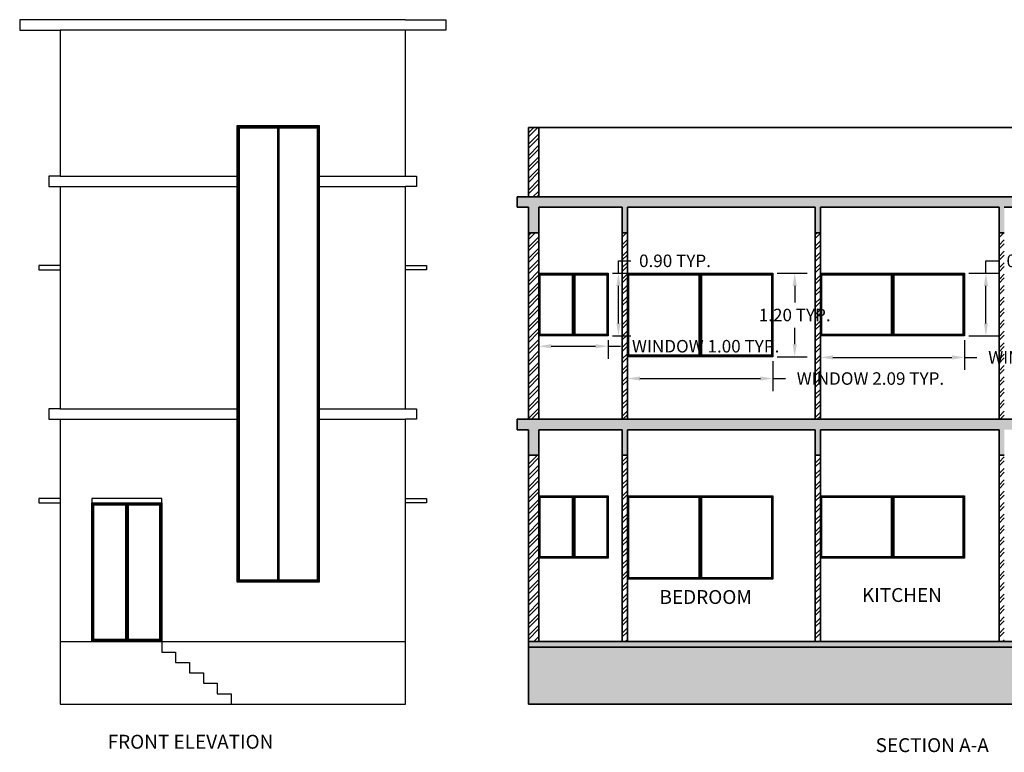
# Model space of a CAD drawing. Units: metres. Extents: x 8.1 to 56.2, y -9.3 to 36.3.
# Tile 3 of 6: x 8.3 to 22.5, y 25.7 to 36.3. Entities that reach past the tile are written whole.
import ezdxf

# ---------------------------------------------------------------- set-up
doc = ezdxf.new("R2010")
doc.units = ezdxf.units.M
doc.header["$LTSCALE"] = 0.01
doc.header["$MEASUREMENT"] = 0
for name, color, linetype, lineweight in [('A-ANNO-DIMS', 2, 'Continuous', 18), ('A-ANNO-TEXT', 7, 'Continuous', 18), ('A-ELEV', 7, 'Continuous', 25), ('A-GLAZ', 3, 'Continuous', 25), ('A-SECT', 7, 'Continuous', 35), ('A-SECT-PATT', 8, 'Continuous', 13)]:
    doc.layers.add(name, color=color, linetype=linetype, lineweight=lineweight)
doc.styles.get("Standard").update_dxf_attribs({"font": 'arial.ttf'})
doc.dimstyles.get("Standard").update_dxf_attribs({"dimtxt": 0.18, "dimasz": 0.18, "dimexe": 0.18, "dimexo": 0.0625, "dimgap": 0.09, "dimtad": 0, "dimtih": 1, "dimtoh": 1, "dimzin": 0, "dimdsep": 46, "dimtxsty": 'Standard', "dimcen": 0.09, "dimadec": 0, "dimazin": 0, "dimtfac": 1, "dimtofl": 0, "dimtmove": 0, "dimatfit": 3, "dimfxl": 1, "dimtolj": 1, "dimtzin": 0, "dimarcsym": 0})
pattern_1 = [(0, (-2.197816, 0), (0.023, 0.023), [0.0115, -0.0345]), (90, (-2.192066, -0.00575), (-0.023, 0.023), [0.0115, -0.0345])]
pattern_2 = [(45, (-2.19782, 0), (-0.08220116, 0.08220116), []), (45, (-2.14301, 0), (-0.08220116, 0.08220116), [])]

# ---------------------------------------------------------------- blocks, each defined once
blk = doc.blocks.new('WIN-1000')
for p, q in [((0.479, 0.88), (0.479, 0.02)), ((0.489, 0.88), (0.489, 0.02)), ((0.499, 0.88), (0.499, 0.02)), ((0.509, 0.88), (0.509, 0.02)), ((0.519, 0.88), (0.519, 0.02))]:
    blk.add_line(p, q)
for points in [[(0, 0.9), (0.997, 0.9), (0.997, 0), (0, 0)], [(0.01, 0.89), (0.987, 0.89), (0.987, 0.01), (0.01, 0.01)], [(0.02, 0.88), (0.977, 0.88), (0.977, 0.02), (0.02, 0.02)]]:
    blk.add_lwpolyline(points, close=True)
blk = doc.blocks.new('WIN-2100')
for p, q in [((1.026, 1.18), (1.026, 0.02)), ((1.036, 1.18), (1.036, 0.02)), ((1.046, 1.18), (1.046, 0.02)), ((1.056, 1.18), (1.056, 0.02)), ((1.066, 1.18), (1.066, 0.02))]:
    blk.add_line(p, q)
for points in [[(0, 1.2), (2.092, 1.2), (2.092, 0), (0, 0)], [(0.01, 1.19), (2.082, 1.19), (2.082, 0.01), (0.01, 0.01)], [(0.02, 1.18), (2.072, 1.18), (2.072, 0.02), (0.02, 0.02)]]:
    blk.add_lwpolyline(points, close=True)
blk = doc.blocks.new('WIN-2100X900')
for p, q in [((1.016, 0.88), (1.016, 0.02)), ((1.026, 0.88), (1.026, 0.02)), ((1.036, 0.88), (1.036, 0.02)), ((1.046, 0.88), (1.046, 0.02)), ((1.056, 0.88), (1.056, 0.02))]:
    blk.add_line(p, q)
for points in [[(0, 0.9), (2.071, 0.9), (2.071, 0), (0, 0)], [(0.01, 0.89), (2.061, 0.89), (2.061, 0.01), (0.01, 0.01)], [(0.02, 0.88), (2.051, 0.88), (2.051, 0.02), (0.02, 0.02)]]:
    blk.add_lwpolyline(points, close=True)
blk = doc.blocks.new('*D33')
at = {"layer": 'A-ANNO-DIMS', "color": 0, "lineweight": -2, "ltscale": 0.01, "transparency": 16777216}
for p, q in [((15.813, 31.647), (15.813, 31.38)), ((16.81, 31.647), (16.81, 31.38)), ((15.993, 31.56), (16.63, 31.56)), ((16.81, 31.56), (16.99, 31.56))]:
    blk.add_line(p, q, dxfattribs=at)
at = {"layer": 'A-ANNO-DIMS', "color": 0, "ltscale": 0.01, "transparency": 16777216}
for points in [[(15.993, 31.59), (15.993, 31.53), (15.813, 31.56)], [(16.63, 31.59), (16.63, 31.53), (16.81, 31.56)]]:
    blk.add_solid(points, dxfattribs=at)
at = {"layer": 'Defpoints', "color": 0, "ltscale": 0.01, "transparency": 16777216}
for p in [(15.813, 31.709), (16.81, 31.709), (16.81, 31.56)]:
    blk.add_point(p, dxfattribs=at)
at = {"layer": 'A-ANNO-DIMS', "color": 0, "ltscale": 0.01, "transparency": 16777216, "insert": (18.213, 31.56), "char_height": 0.18, "attachment_point": 5}
blk.add_mtext('\\A1;WINDOW 1.00 TYP.', dxfattribs=at)
blk = doc.blocks.new('*D34')
at = {"layer": 'A-ANNO-DIMS', "color": 0, "lineweight": -2, "ltscale": 0.01, "transparency": 16777216}
for p, q in [((16.959, 32.609), (16.959, 32.789)), ((16.959, 32.789), (17.139, 32.789)), ((16.872, 32.609), (17.139, 32.609)), ((16.959, 31.889), (16.959, 32.429)), ((16.872, 31.709), (17.139, 31.709))]:
    blk.add_line(p, q, dxfattribs=at)
at = {"layer": 'A-ANNO-DIMS', "color": 0, "ltscale": 0.01, "transparency": 16777216}
for points in [[(16.929, 32.429), (16.989, 32.429), (16.959, 32.609)], [(16.929, 31.889), (16.989, 31.889), (16.959, 31.709)]]:
    blk.add_solid(points, dxfattribs=at)
at = {"layer": 'Defpoints', "color": 0, "ltscale": 0.01, "transparency": 16777216}
for p in [(16.81, 32.609), (16.959, 32.609), (16.81, 31.709)]:
    blk.add_point(p, dxfattribs=at)
at = {"layer": 'A-ANNO-DIMS', "color": 0, "ltscale": 0.01, "transparency": 16777216, "insert": (17.772, 32.789), "char_height": 0.18, "attachment_point": 5}
blk.add_mtext('\\A1;0.90 TYP.', dxfattribs=at)
blk = doc.blocks.new('*D35')
at = {"layer": 'A-ANNO-DIMS', "color": 0, "lineweight": -2, "ltscale": 0.01, "transparency": 16777216}
for p, q in [((17.088, 31.347), (17.088, 30.915)), ((19.18, 31.347), (19.18, 30.915)), ((17.268, 31.095), (19, 31.095)), ((19.18, 31.095), (19.36, 31.095))]:
    blk.add_line(p, q, dxfattribs=at)
at = {"layer": 'A-ANNO-DIMS', "color": 0, "ltscale": 0.01, "transparency": 16777216}
for points in [[(17.268, 31.125), (17.268, 31.065), (17.088, 31.095)], [(19, 31.125), (19, 31.065), (19.18, 31.095)]]:
    blk.add_solid(points, dxfattribs=at)
at = {"layer": 'Defpoints', "color": 0, "ltscale": 0.01, "transparency": 16777216}
for p in [(17.088, 31.409), (19.18, 31.409), (19.18, 31.095)]:
    blk.add_point(p, dxfattribs=at)
at = {"layer": 'A-ANNO-DIMS', "color": 0, "ltscale": 0.01, "transparency": 16777216, "insert": (20.583, 31.095), "char_height": 0.18, "attachment_point": 5}
blk.add_mtext('\\A1;WINDOW 2.09 TYP.', dxfattribs=at)
blk = doc.blocks.new('*D36')
at = {"layer": 'A-ANNO-DIMS', "color": 0, "lineweight": -2, "ltscale": 0.01, "transparency": 16777216}
for p, q in [((19.243, 32.609), (19.674, 32.609)), ((19.494, 32.429), (19.494, 32.191)), ((19.494, 31.589), (19.494, 31.827)), ((19.243, 31.409), (19.674, 31.409))]:
    blk.add_line(p, q, dxfattribs=at)
at = {"layer": 'A-ANNO-DIMS', "color": 0, "ltscale": 0.01, "transparency": 16777216}
for points in [[(19.464, 32.429), (19.524, 32.429), (19.494, 32.609)], [(19.464, 31.589), (19.524, 31.589), (19.494, 31.409)]]:
    blk.add_solid(points, dxfattribs=at)
at = {"layer": 'Defpoints', "color": 0, "ltscale": 0.01, "transparency": 16777216}
for p in [(19.18, 32.609), (19.494, 32.609), (19.18, 31.409)]:
    blk.add_point(p, dxfattribs=at)
at = {"layer": 'A-ANNO-DIMS', "color": 0, "ltscale": 0.01, "transparency": 16777216, "insert": (19.494, 32.009), "char_height": 0.18, "attachment_point": 5}
blk.add_mtext('\\A1;1.20 TYP.', dxfattribs=at)
blk = doc.blocks.new('*D37')
at = {"layer": 'A-ANNO-DIMS', "color": 0, "lineweight": -2, "ltscale": 0.01, "transparency": 16777216}
for p, q in [((19.863, 31.647), (19.863, 31.219)), ((21.934, 31.647), (21.934, 31.219)), ((20.043, 31.399), (21.754, 31.399)), ((21.934, 31.399), (22.114, 31.399))]:
    blk.add_line(p, q, dxfattribs=at)
at = {"layer": 'A-ANNO-DIMS', "color": 0, "ltscale": 0.01, "transparency": 16777216}
for points in [[(20.043, 31.429), (20.043, 31.369), (19.863, 31.399)], [(21.754, 31.429), (21.754, 31.369), (21.934, 31.399)]]:
    blk.add_solid(points, dxfattribs=at)
at = {"layer": 'Defpoints', "color": 0, "ltscale": 0.01, "transparency": 16777216}
for p in [(19.863, 31.709), (21.934, 31.709), (21.934, 31.399)]:
    blk.add_point(p, dxfattribs=at)
at = {"layer": 'A-ANNO-DIMS', "color": 0, "ltscale": 0.01, "transparency": 16777216, "insert": (23.337, 31.399), "char_height": 0.18, "attachment_point": 5}
blk.add_mtext('\\A1;WINDOW 2.07 TYP.', dxfattribs=at)
blk = doc.blocks.new('*D38')
at = {"layer": 'A-ANNO-DIMS', "color": 0, "lineweight": -2, "ltscale": 0.01, "transparency": 16777216}
for p, q in [((22.244, 32.609), (22.244, 32.789)), ((22.244, 32.789), (22.424, 32.789)), ((21.996, 32.609), (22.424, 32.609)), ((22.244, 31.889), (22.244, 32.429)), ((21.996, 31.709), (22.424, 31.709))]:
    blk.add_line(p, q, dxfattribs=at)
at = {"layer": 'A-ANNO-DIMS', "color": 0, "ltscale": 0.01, "transparency": 16777216}
for points in [[(22.214, 32.429), (22.274, 32.429), (22.244, 32.609)], [(22.214, 31.889), (22.274, 31.889), (22.244, 31.709)]]:
    blk.add_solid(points, dxfattribs=at)
at = {"layer": 'Defpoints', "color": 0, "ltscale": 0.01, "transparency": 16777216}
for p in [(21.934, 32.609), (22.244, 32.609), (21.934, 31.709)]:
    blk.add_point(p, dxfattribs=at)
at = {"layer": 'A-ANNO-DIMS', "color": 0, "ltscale": 0.01, "transparency": 16777216, "insert": (23.057, 32.789), "char_height": 0.18, "attachment_point": 5}
blk.add_mtext('\\A1;0.90 TYP.', dxfattribs=at)

msp = doc.modelspace()

# ---------------------------------------------------------------- hatches: boundary and pattern name
at = {"layer": 'A-SECT-PATT'}
h = msp.add_hatch(dxfattribs=at)
h.set_pattern_fill('ANSI32', color=256, scale=0.31)
h.set_pattern_definition(pattern_2)
h.paths.add_polyline_path([(15.813, 33.192), (15.663, 33.192), (15.663, 30.509), (15.813, 30.509)])
h.paths.add_polyline_path([(17.013, 30.509), (17.088, 30.509), (17.088, 33.192), (17.013, 33.192)])
h.paths.add_polyline_path([(15.663, 33.709), (15.813, 33.709), (15.813, 34.709), (15.663, 34.709)])
h = msp.add_hatch(dxfattribs=at)
h.set_pattern_fill('CROSS', color=256, scale=0.094)
h.set_pattern_definition([(0, (-2.197816, 0), (0.0235, 0.0235), [0.01175, -0.03525]), (90, (-2.19194, -0.005875), (-0.0235, 0.0235), [0.01175, -0.03525])])
h.paths.add_polyline_path([(15.663, 33.709), (15.503, 33.709), (15.503, 33.559), (15.663, 33.559), (15.663, 33.192), (15.813, 33.192), (15.813, 33.559), (17.013, 33.559), (17.013, 33.192), (17.088, 33.192), (17.088, 33.559), (19.788, 33.559), (19.788, 33.192), (19.863, 33.192), (19.863, 33.559), (22.433, 33.559), (22.433, 33.192), (22.508, 33.192), (22.508, 33.559), (25.558, 33.559), (25.558, 33.192), (25.633, 33.192), (25.633, 33.559), (27.733, 33.559), (27.733, 33.192), (27.883, 33.192), (27.883, 33.559), (28.044, 33.559), (28.044, 33.709), (27.883, 33.709)])
h = msp.add_hatch(dxfattribs=at)
h.set_pattern_fill('ANSI32', color=256, scale=0.31)
h.set_pattern_definition(pattern_2)
h.paths.add_polyline_path([(19.863, 33.192), (19.788, 33.192), (19.788, 30.509), (19.863, 30.509)])
h.paths.add_polyline_path([(22.508, 33.192), (22.433, 33.192), (22.433, 30.509), (22.508, 30.509)])
h.paths.add_polyline_path([(25.633, 33.192), (25.558, 33.192), (25.558, 30.509), (25.633, 30.509)])
h.paths.add_polyline_path([(27.883, 33.192), (27.733, 33.192), (27.733, 30.509), (27.883, 30.509)])
h.paths.add_polyline_path([(27.733, 27.309), (27.883, 27.309), (27.883, 29.992), (27.733, 29.992)])
h.paths.add_polyline_path([(25.558, 27.309), (25.633, 27.309), (25.633, 29.992), (25.558, 29.992)])
h = msp.add_hatch(dxfattribs=at)
h.set_pattern_fill('CROSS', color=256, scale=0.092)
h.set_pattern_definition(pattern_1)
h.paths.add_polyline_path([(17.013, 30.359), (17.013, 29.992), (17.088, 29.992), (17.088, 30.359), (19.788, 30.359), (19.788, 29.992), (19.863, 29.992), (19.863, 30.359), (22.433, 30.359), (22.433, 29.992), (22.508, 29.992), (22.508, 30.359), (25.558, 30.359), (25.558, 29.992), (25.633, 29.992), (25.633, 30.359), (27.733, 30.359), (27.733, 29.992), (27.883, 29.992), (27.883, 30.359), (28.044, 30.359), (28.044, 30.509), (27.883, 30.509), (15.663, 30.509), (15.503, 30.509), (15.503, 30.359), (15.663, 30.359), (15.663, 29.992), (15.813, 29.992), (15.813, 30.359)])
h = msp.add_hatch(dxfattribs=at)
h.set_pattern_fill('ANSI32', color=256, scale=0.31)
h.set_pattern_definition(pattern_2)
h.paths.add_polyline_path([(22.433, 27.309), (22.508, 27.309), (22.508, 29.992), (22.433, 29.992)])
h.paths.add_polyline_path([(19.788, 27.309), (19.863, 27.309), (19.863, 29.992), (19.788, 29.992)])
h.paths.add_polyline_path([(17.013, 27.309), (17.088, 27.309), (17.088, 29.992), (17.013, 29.992)])
h.paths.add_polyline_path([(15.663, 27.309), (15.813, 27.309), (15.813, 29.992), (15.663, 29.992)])
h = msp.add_hatch(dxfattribs=at)
h.set_pattern_fill('CROSS', color=256, scale=0.092)
h.set_pattern_definition(pattern_1)
h.paths.add_polyline_path([(15.663, 27.309), (15.663, 27.229), (27.883, 27.229), (27.883, 27.309)])
h = msp.add_hatch(dxfattribs=at)
h.set_pattern_fill('GRAVEL', color=256, scale=0.7)
h.set_pattern_definition([(228.01279, (-1.693816, 0.7), (-5.6, -6.3), [0.094175, -9.323362]), (184.96974, (-1.756816, 0.63), (8.4, 0.7), [0.161608, -15.999147]), (132.51045, (-1.917816, 0.616), (7, -7.7), [0.113952, -11.281223]), (267.27369, (-2.190816, 0.441), (0.7, 14), [0.147167, -14.569491]), (292.83365, (-2.197816, 0.294), (-3.5, 8.4), [0.1443085, -14.286561]), (357.27369, (-2.141816, 0.161), (-14, 0.7), [0.147167, -14.569491]), (37.69424, (-1.994816, 0.154), (-9.1, -7), [0.19462, -19.267394]), (72.25533, (-1.840816, 0.273), (4.9, 15.4), [0.183742, -18.190425]), (121.42957, (-1.784816, 0.448), (-5.6, 9.1), [0.147665, -14.618851]), (175.23636, (-1.861816, 0.574), (7.7, -0.7), [0.168582, -8.260534]), (222.39744, (-2.029816, 0.588), (-8.4, -7.7), [0.2180136, -21.5833625]), (138.81407, (-1.497816, 0.434), (-4.9, 4.2), [0.074411, -7.366691]), (171.46923, (-1.553816, 0.483), (9.1, -1.4), [0.141566, -14.015058]), (225, (-1.6938, 0.504), (-1e-16, -0.7), [0.098995, -0.890955]), (203.1986, (-1.74282, 0.588), (3.5, 1.4), [0.053311, -5.277731]), (291.8014, (-1.79182, 0.567), (-0.7, 2.1), [0.075392, -3.694223]), (30.96376, (-1.76382, 0.497), (2.1, 1.4), [0.12245, -3.959216]), (161.56505, (-1.65882, 0.56), (1.4, -0.7), [0.088544, -2.125051]), (16.38954, (-2.197816, 0.567), (7, 2.1), [0.12404, -12.279992]), (70.34618, (-2.078816, 0.602), (-2.8, -7.7), [0.104063, -10.302185]), (293.1986, (-1.65882, 0.7), (-1.4, 3.5), [0.10662, -5.224421]), (343.61046, (-1.616816, 0.602), (-7, 2.1), [0.12404, -12.279992]), (339.44395, (-2.197816, 0.133), (-3.5, 1.4), [0.119616, -5.861187]), (294.77514, (-2.085816, 0.091), (-3.5, 7.7), [0.100225, -9.92225]), (66.8014, (-1.65182, 0), (1.4, 3.5), [0.10662, -5.224421]), (17.35402, (-1.609816, 0.098), (-9.1, -2.8), [0.117342, -11.616797]), (69.44395, (-1.994816, 0), (-1.4, -3.5), [0.059808, -5.920995]), (101.30993, (-1.69382, 0), (-0.7, 2.8), [0.035693, -3.533621]), (165.96376, (-1.70082, 0.035), (2.1, -0.7), [0.144309, -2.741865]), (186.00901, (-1.840816, 0.07), (7, 0.7), [0.133735, -13.239746]), (303.69007, (-1.76382, 0.434), (-0.7, 1.4), [0.100955, -2.42293]), (353.15723, (-1.707816, 0.35), (11.9, -1.4), [0.176256, -17.449294]), (60.9454, (-1.532816, 0.329), (-2.8, -4.9), [0.072069, -7.134872]), (90, (-1.4978, 0.392), (-0.7, 0.7), [0.042, -0.658]), (120.25644, (-1.854816, 0.091), (2.8, -4.9), [0.097247, -9.627464]), (48.01279, (-1.903816, 0.175), (5.6, 6.3), [0.18835, -9.229186]), (0, (-1.7778, 0.315), (0.7, 0.7), [0.182, -0.518]), (325.30485, (-1.595816, 0.315), (7, -4.9), [0.11068, -10.957292]), (254.0546, (-1.50482, 0.252), (-0.7, -2.8), [0.101921, -4.994156]), (207.645975, (-1.532816, 0.154), (-13.3, -7), [0.1659455, -16.428632]), (175.42608, (-1.679816, 0.077), (-9.1, 0.7), [0.175559, -17.380351])])
h.paths.add_polyline_path([(27.883, 26.409), (27.883, 27.229), (15.663, 27.229), (15.663, 26.409)])

# ---------------------------------------------------------------- linework, layer by layer
at = {"layer": 'A-ELEV'}
for p, q in [((8.606, 36.259), (8.347, 36.259)), ((8.347, 36.259), (8.347, 36.109)), ((8.927, 36.259), (8.606, 36.259)), ((13.894, 36.259), (8.927, 36.259)), ((13.894, 36.259), (14.216, 36.259)), ((14.216, 36.259), (14.475, 36.259)), ((14.475, 36.259), (14.475, 36.109)), ((8.347, 36.109), (8.606, 36.109)), ((8.606, 36.109), (8.927, 36.109)), ((8.927, 36.109), (8.927, 34.009)), ((13.894, 36.109), (8.927, 36.109)), ((13.894, 34.009), (13.894, 36.109)), ((14.216, 36.109), (13.894, 36.109)), ((14.475, 36.109), (14.216, 36.109)), ((12.056, 34.705), (12.056, 28.194)), ((12.066, 34.705), (12.066, 28.194)), ((12.076, 34.705), (12.076, 28.194)), ((8.927, 34.009), (8.767, 34.009)), ((8.767, 34.009), (8.767, 33.859)), ((8.927, 34.009), (11.477, 34.009)), ((12.656, 34.009), (13.894, 34.009)), ((13.894, 34.009), (14.055, 34.009)), ((14.055, 34.009), (14.055, 33.859)), ((8.767, 33.859), (8.927, 33.859)), ((8.927, 33.859), (11.477, 33.859)), ((8.927, 33.859), (8.927, 30.659)), ((12.656, 33.859), (13.894, 33.859)), ((13.894, 30.659), (13.894, 33.859)), ((14.055, 33.859), (13.894, 33.859)), ((8.927, 32.72), (8.623, 32.72)), ((8.623, 32.72), (8.623, 32.658)), ((13.894, 32.72), (14.198, 32.72)), ((14.198, 32.72), (14.198, 32.658)), ((8.623, 32.658), (8.927, 32.658)), ((14.198, 32.658), (13.894, 32.658)), ((8.927, 30.659), (8.767, 30.659)), ((8.767, 30.659), (8.767, 30.509)), ((8.927, 30.659), (11.477, 30.659)), ((12.656, 30.659), (13.894, 30.659)), ((13.894, 30.659), (14.055, 30.659)), ((14.055, 30.659), (14.055, 30.509)), ((8.767, 30.509), (8.927, 30.509)), ((8.927, 30.509), (11.477, 30.509)), ((8.927, 30.509), (8.927, 27.309)), ((12.656, 30.509), (13.894, 30.509)), ((13.894, 27.309), (13.894, 30.509)), ((14.055, 30.509), (13.894, 30.509)), ((8.927, 29.37), (8.623, 29.37)), ((8.623, 29.37), (8.623, 29.308)), ((13.894, 29.37), (14.198, 29.37)), ((14.198, 29.37), (14.198, 29.308)), ((8.623, 29.308), (8.927, 29.308)), ((9.867, 29.278), (9.867, 27.339)), ((9.877, 29.278), (9.877, 27.339)), ((9.887, 29.278), (9.887, 27.339)), ((9.897, 29.278), (9.897, 27.339)), ((9.907, 29.278), (9.907, 27.339)), ((14.198, 29.308), (13.894, 29.308)), ((8.927, 27.309), (13.894, 27.309)), ((8.927, 27.309), (8.927, 26.409)), ((10.389, 27.309), (10.389, 27.159)), ((13.894, 26.409), (13.894, 27.309)), ((10.389, 27.159), (10.589, 27.159)), ((10.589, 27.159), (10.589, 27.009)), ((10.589, 27.009), (10.789, 27.009)), ((10.789, 27.009), (10.789, 26.859)), ((10.789, 26.859), (10.989, 26.859)), ((10.989, 26.859), (10.989, 26.709)), ((10.989, 26.709), (11.189, 26.709)), ((11.189, 26.709), (11.189, 26.559)), ((11.189, 26.559), (11.389, 26.559)), ((11.389, 26.559), (11.389, 26.409)), ((8.927, 26.409), (13.894, 26.409))]:
    msp.add_line(p, q, dxfattribs=at)
for points in [[(11.477, 34.735), (12.656, 34.735), (12.656, 28.164), (11.477, 28.164)], [(11.487, 34.725), (12.646, 34.725), (12.646, 28.174), (11.487, 28.174)], [(11.497, 34.715), (12.636, 34.715), (12.636, 28.184), (11.497, 28.184)], [(11.507, 34.705), (12.626, 34.705), (12.626, 28.194), (11.507, 28.194)], [(9.385, 29.308), (10.389, 29.308), (10.389, 29.37), (9.385, 29.37)], [(10.389, 27.309), (9.385, 27.309), (9.385, 29.308), (10.389, 29.308)], [(10.379, 27.319), (9.395, 27.319), (9.395, 29.298), (10.379, 29.298)], [(10.369, 27.329), (9.405, 27.329), (9.405, 29.288), (10.369, 29.288)], [(10.359, 27.339), (9.415, 27.339), (9.415, 29.278), (10.359, 29.278)]]:
    msp.add_lwpolyline(points, close=True, dxfattribs=at)
at = {"layer": 'A-SECT'}
for p, q in [((15.663, 34.709), (25.701, 34.709)), ((15.663, 33.709), (15.663, 34.709)), ((15.813, 33.709), (15.813, 34.709)), ((15.663, 33.709), (15.503, 33.709)), ((15.503, 33.709), (15.503, 33.559)), ((15.663, 33.709), (27.883, 33.709)), ((15.503, 33.559), (15.663, 33.559)), ((15.663, 30.509), (15.663, 33.559)), ((15.813, 33.559), (17.013, 33.559)), ((15.813, 30.509), (15.813, 33.559)), ((17.013, 30.509), (17.013, 33.559)), ((17.088, 30.509), (17.088, 33.559)), ((17.088, 33.559), (19.788, 33.559)), ((19.788, 30.509), (19.788, 33.559)), ((19.863, 30.509), (19.863, 33.559)), ((19.863, 33.559), (22.433, 33.559)), ((22.433, 30.509), (22.433, 33.559)), ((22.508, 33.559), (25.558, 33.559)), ((15.663, 33.192), (15.813, 33.192)), ((17.013, 33.192), (17.088, 33.192)), ((19.788, 33.192), (19.863, 33.192)), ((22.433, 33.192), (22.508, 33.192)), ((15.663, 30.509), (15.503, 30.509)), ((15.503, 30.509), (15.503, 30.359)), ((15.663, 30.509), (27.883, 30.509)), ((15.503, 30.359), (15.663, 30.359)), ((15.663, 27.309), (15.663, 30.359)), ((15.813, 30.359), (17.013, 30.359)), ((15.813, 27.309), (15.813, 30.359)), ((17.013, 27.309), (17.013, 30.359)), ((17.088, 27.309), (17.088, 30.359)), ((17.088, 30.359), (19.788, 30.359)), ((19.788, 27.309), (19.788, 30.359)), ((19.863, 27.309), (19.863, 30.359)), ((19.863, 30.359), (22.433, 30.359)), ((22.433, 27.309), (22.433, 30.359)), ((15.663, 29.992), (15.813, 29.992)), ((17.013, 29.992), (17.088, 29.992)), ((19.788, 29.992), (19.863, 29.992)), ((22.433, 29.992), (22.508, 29.992)), ((15.663, 27.309), (27.883, 27.309)), ((15.663, 26.409), (15.663, 27.309)), ((15.663, 27.229), (27.883, 27.229)), ((15.663, 26.409), (27.883, 26.409))]:
    msp.add_line(p, q, dxfattribs=at)

# ---------------------------------------------------------------- block references
at = {"layer": 'A-GLAZ'}
for name, p in [('WIN-1000', (15.813, 31.709)), ('WIN-2100', (17.088, 31.409)), ('WIN-2100X900', (19.863, 31.709)), ('WIN-1000', (15.813, 28.509)), ('WIN-2100', (17.088, 28.209)), ('WIN-2100X900', (19.863, 28.509))]:
    msp.add_blockref(name, p, dxfattribs=at)

# ---------------------------------------------------------------- texts
at = {"layer": 'A-ANNO-TEXT', "char_height": 0.2, "attachment_point": 1}
for s, width, insert in [('\\pxqc;BEDROOM', 1.61769, (17.404, 28.051)), ('\\pxqc;KITCHEN', 1.61769, (20.227, 28.08)), ('\\pxqc;FRONT ELEVATION', 4.05553, (8.776, 25.968)), ('\\pxqc;SECTION A-A', 4.05553, (19.444, 25.919))]:
    msp.add_mtext_dynamic_manual_height_columns(s, width=width, gutter_width=1, heights=[0], dxfattribs=dict(at, insert=insert))

# ---------------------------------------------------------------- dimensions: what is measured, and where the dimension line sits
at = {"layer": 'A-ANNO-DIMS', "ltscale": 0.01}
for base, p1, p2, picture, middle in [((16.959, 32.609), (16.81, 31.709), (16.81, 32.609), '*D34', (17.772, 32.789)), ((22.244, 32.609), (21.934, 31.709), (21.934, 32.609), '*D38', (23.057, 32.789)), ((19.494, 32.609), (19.18, 31.409), (19.18, 32.609), '*D36', (19.494, 32.009))]:
    dim = msp.add_linear_dim(base=base, p1=p1, p2=p2, angle=90, text='<> TYP.', dimstyle='Standard', override={"dimdec": 2, "dimrnd": 0, "dimzin": 0, "dimlunit": 2}, dxfattribs=at)
    dim.commit()
    dim.dimension.update_dxf_attribs({"geometry": picture, "text_midpoint": middle})
for base, p1, p2, picture, middle in [((16.81, 31.56), (15.813, 31.709), (16.81, 31.709), '*D33', (18.213, 31.56)), ((21.934, 31.399), (19.863, 31.709), (21.934, 31.709), '*D37', (23.337, 31.399)), ((19.18, 31.095), (17.088, 31.409), (19.18, 31.409), '*D35', (20.583, 31.095))]:
    dim = msp.add_linear_dim(base=base, p1=p1, p2=p2, text='WINDOW <> TYP.', dimstyle='Standard', override={"dimdec": 2, "dimrnd": 0, "dimzin": 0, "dimlunit": 2}, dxfattribs=at)
    dim.commit()
    dim.dimension.update_dxf_attribs({"geometry": picture, "text_midpoint": middle})

doc.saveas('drawing.dxf')
